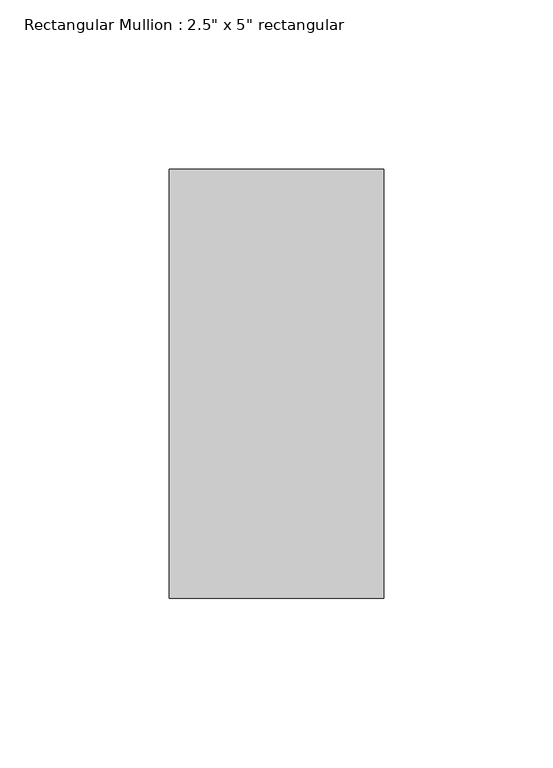
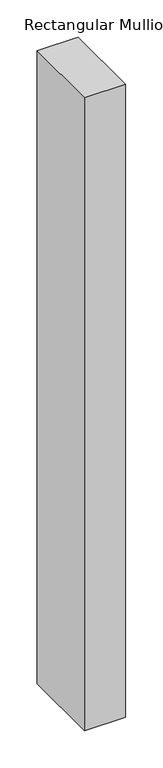
"""IFC4 building model written with IfcOpenShell, lengths in millimetres: member geometry."""

from ifc_helpers import new_model, si_unit, frame, origin, place, context, project, spatial, polyline, outline, extrude, source, transform, mapped, element, save


def member_6ef8dc49(model_context):
    return source(origin(), model_context, "Body", "SweptSolid", [
        extrude(outline(polyline([(0.0, 63.5), (0.0, -63.5), (-63.5, -63.5), (-63.5, 63.5), (0.0, 63.5)])), frame((0.0, 0.0, -1035.05), z_axis=(0.0, 0.0, 1.0), x_axis=(1.0, 0.0, 0.0)), (0.0, 0.0, 1.0), 1035.05),
    ])


if __name__ == "__main__":
    model = new_model("IFC4")
    model_context = context("Model", 3, world=origin())
    ifc_project = project(units=[si_unit("LENGTHUNIT", "METRE", prefix="MILLI")], contexts=[model_context])
    site = spatial("IfcSite", under=ifc_project)
    building = spatial("IfcBuilding", under=site)
    placement = place(None, origin())
    member_shape = member_6ef8dc49(model_context)
    element("IfcMember", 1, ObjectType="Rectangular Mullion : 2.5\" x 5\" rectangular", at=placement, inside=building, context=model_context, shape_type="MappedRepresentation", body=[
        mapped(member_shape, transform((0.0, 0.0, 0.0), x_axis=(1.0, 0.0, 0.0), y_axis=(0.0, 1.0, 0.0), z_axis=(0.0, 0.0, 1.0))),
    ])
    save(model, "model.ifc")

# Revit data of these elements
# Type "Rectangular Mullion : 2.5\" x 5\" rectangular"
#   built-in parameter 1007304 = 0.416667 (stored number, unit not read)
#   built-in parameter 1007301 = 0.104167 (stored number, unit not read)
#   built-in parameter 1007300 = 0.104167 (stored number, unit not read)
# Element 1 (IfcMember, "Rectangular Mullion : 2.5\" x 5\" rectangular")
#   Materials on its faces: "Aluminum"
# Materials
#   "Aluminum": class "Metal", colour RGB 247 247 247, transparency 0, Description = "Aluminum 6061", Cost = 0
